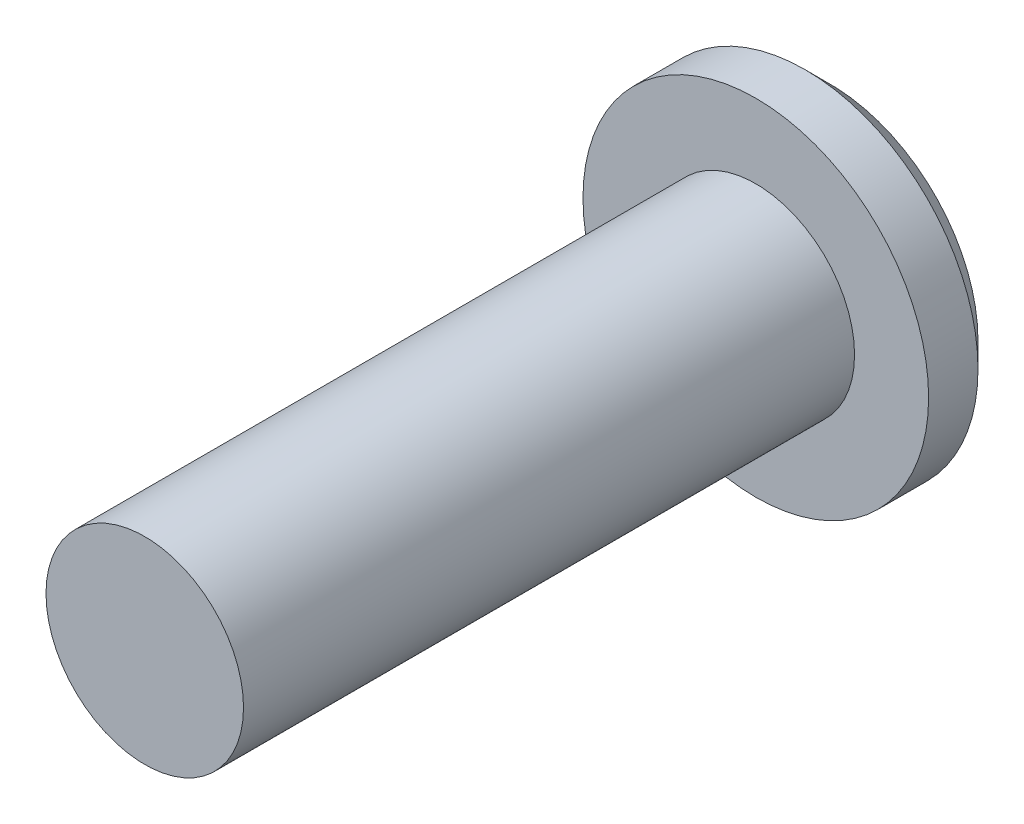
SolidWorks part; units mm, degrees
material "Plain Carbon Steel"
ref_plane "Front Plane" through (0, 0, 0) normal (0, 0, 1) x (1, 0, 0)
ref_plane "Top Plane" through (0, 0, 0) normal (0, 1, 0) x (1, 0, 0)
ref_plane "Right Plane" through (0, 0, 0) normal (1, 0, 0) x (0, 0, -1)
sketch "Head Profile Ø14" plane through (0, 0, 0) normal (0, 0, 1) x (1, 0, 0)
  circle A0 centre (0, 0) radius 7
  dimension "D1" = 14
extrude "Head Ø14x3" add sketch "Head Profile Ø14" along normal blind 3
sketch "Shank Profile Ø8" plane through (0, 0, 3) normal (0, 0, 1) x (1, 0, 0)
  circle A0 centre (0, 0) radius 4
  dimension "D1" = 8
extrude "Shank Ø8x24.75" add sketch "Shank Profile Ø8" along normal blind 24.75
cosmetic thread "Cosmetic Thread1" parameters "D1"=3, "D2"=6.561
chamfer "Head Chamfer 1x45°" distance 1 angle 45 1 edges at (7, 0, 0)
